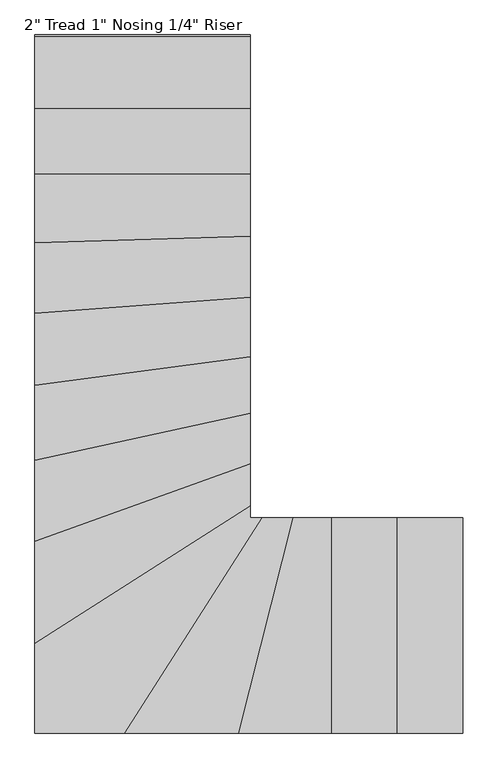
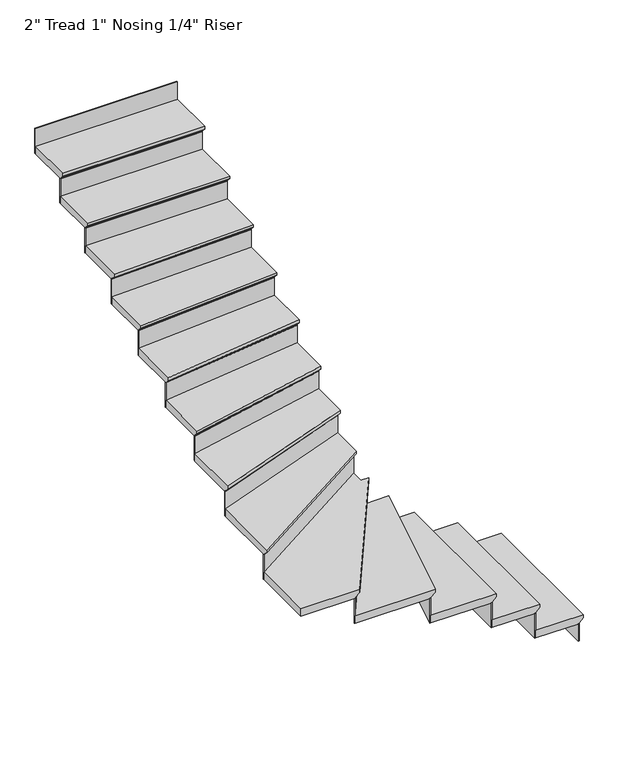
"""IFC4 building model written with IfcOpenShell, lengths in millimetres: stair flight geometry."""

from ifc_helpers import new_model, si_unit, origin, place, context, project, spatial, faceted_brep, source, transform, mapped, element, save


def stair_flight_14253777(model_context):
    return source(origin(), model_context, "Body", "Brep", [
        faceted_brep([(-4378.4230036, -1246.1564015, 10428.8166667), (-4378.4230036, -1246.1564015, 10447.8666667), (-4378.4230036, -2160.5564015, 10447.8666667), (-4378.4230036, -2160.5564015, 10428.8166667), (-4403.8230036, -1246.1564015, 10403.4166667), (-4403.8230036, -2160.5564015, 10403.4166667), (-4683.2230036, -1246.1564015, 10447.8666667), (-4683.2230036, -2160.5564015, 10447.8666667), (-4403.8230036, -2160.5564015, 10397.0666667), (-4683.2230036, -2160.5564015, 10397.0666667), (-4683.2230036, -1246.1564015, 10397.0666667), (-4403.8230036, -1246.1564015, 10397.0666667)], [[[0, 1, 2, 3]], [[4, 0, 3, 5]], [[2, 1, 6, 7]], [[8, 9, 10, 11]], [[2, 7, 9, 8, 5, 3]], [[8, 11, 4, 5]], [[6, 1, 0, 4, 11, 10]], [[7, 6, 10, 9]]]),
        faceted_brep([(-4403.8230036, -1246.1564015, 10397.0666667), (-4403.8230036, -1246.1564015, 10278.5333333), (-4410.1730036, -1246.1564015, 10278.5333333), (-4410.1730036, -1246.1564015, 10397.0666667), (-4403.8230036, -2160.5564015, 10397.0666667), (-4410.1730036, -2160.5564015, 10397.0666667), (-4410.1730036, -2160.5564015, 10278.5333333), (-4403.8230036, -2160.5564015, 10278.5333333)], [[[0, 1, 2, 3]], [[4, 5, 6, 7]], [[1, 0, 4, 7]], [[2, 1, 7, 6]], [[3, 2, 6, 5]], [[0, 3, 5, 4]]]),
        faceted_brep([(-4683.2230036, -1246.1564015, 10566.4), (-4683.2230036, -1246.1564015, 10397.0666667), (-4689.5730036, -1246.1564015, 10397.0666667), (-4689.5730036, -1246.1564015, 10566.4), (-4683.2230036, -2160.5564015, 10566.4), (-4689.5730036, -2160.5564015, 10566.4), (-4689.5730036, -2160.5564015, 10397.0666667), (-4683.2230036, -2160.5564015, 10397.0666667)], [[[0, 1, 2, 3]], [[4, 5, 6, 7]], [[1, 0, 4, 7]], [[2, 1, 7, 6]], [[3, 2, 6, 5]], [[0, 3, 5, 4]]]),
        faceted_brep([(-4657.8230036, -2160.5564015, 10617.2), (-4657.8230036, -1246.1564015, 10617.2), (-4962.6230036, -1246.1564015, 10617.2), (-4962.6230036, -2160.5564015, 10617.2), (-4683.2230036, -2160.5564015, 10566.4), (-4962.6230036, -2160.5564015, 10566.4), (-4962.6230036, -1246.1564015, 10566.4), (-4683.2230036, -1246.1564015, 10566.4), (-4683.2230036, -2160.5564015, 10572.75), (-4657.8230036, -2160.5564015, 10598.15), (-4683.2230036, -1246.1564015, 10572.75), (-4657.8230036, -1246.1564015, 10598.15)], [[[0, 1, 2, 3]], [[4, 5, 6, 7]], [[0, 3, 5, 4, 8, 9]], [[4, 7, 10, 8]], [[2, 1, 11, 10, 7, 6]], [[3, 2, 6, 5]], [[11, 1, 0, 9]], [[10, 11, 9, 8]]]),
        faceted_brep([(-4962.6230036, -1246.1564015, 10735.7333333), (-4962.6230036, -1246.1564015, 10566.4), (-4968.9730036, -1246.1564015, 10566.4), (-4968.9730036, -1246.1564015, 10735.7333333), (-4962.6230036, -2160.5564015, 10735.7333333), (-4968.9730036, -2160.5564015, 10735.7333333), (-4968.9730036, -2160.5564015, 10566.4), (-4962.6230036, -2160.5564015, 10566.4)], [[[0, 1, 2, 3]], [[4, 5, 6, 7]], [[1, 0, 4, 7]], [[2, 1, 7, 6]], [[3, 2, 6, 5]], [[0, 3, 5, 4]]]),
        faceted_brep([(-4937.2230036, -2160.5564015, 10786.5333333), (-4937.2230036, -1246.1564015, 10786.5333333), (-5127.3280374, -1246.1564015, 10786.5333333), (-5358.313714, -2160.5564015, 10786.5333333), (-4962.6230036, -2160.5564015, 10735.7333333), (-5358.313714, -2160.5564015, 10735.7333333), (-5127.3280374, -1246.1564015, 10735.7333333), (-4962.6230036, -1246.1564015, 10735.7333333), (-4962.6230036, -2160.5564015, 10742.0833333), (-4937.2230036, -2160.5564015, 10767.4833333), (-4962.6230036, -1246.1564015, 10742.0833333), (-4937.2230036, -1246.1564015, 10767.4833333)], [[[0, 1, 2, 3]], [[4, 5, 6, 7]], [[0, 3, 5, 4, 8, 9]], [[4, 7, 10, 8]], [[2, 1, 11, 10, 7, 6]], [[3, 2, 6, 5]], [[11, 1, 0, 9]], [[10, 11, 9, 8]]]),
        faceted_brep([(-5127.3280374, -1246.1564015, 10905.0666667), (-5127.3280374, -1246.1564015, 10735.7333333), (-5133.8775055, -1246.1564015, 10735.7333333), (-5133.8775055, -1246.1564015, 10905.0666667), (-5358.313714, -2160.5564015, 10905.0666667), (-5364.8631821, -2160.5564015, 10905.0666667), (-5364.8631821, -2160.5564015, 10735.7333333), (-5358.313714, -2160.5564015, 10735.7333333)], [[[0, 1, 2, 3]], [[4, 5, 6, 7]], [[1, 0, 4, 7]], [[2, 1, 7, 6]], [[3, 2, 6, 5]], [[0, 3, 5, 4]]]),
        faceted_brep([(-5332.1158419, -2160.5564015, 10955.8666667), (-5101.1301653, -1246.1564015, 10955.8666667), (-5261.5956265, -1246.1564015, 10955.8666667), (-5846.1950619, -2160.5564015, 10955.8666667), (-5358.313714, -2160.5564015, 10905.0666667), (-5846.1950619, -2160.5564015, 10905.0666667), (-5261.5956265, -1246.1564015, 10905.0666667), (-5127.3280374, -1246.1564015, 10905.0666667), (-5358.313714, -2160.5564015, 10911.4166667), (-5332.1158419, -2160.5564015, 10936.8166667), (-5127.3280374, -1246.1564015, 10911.4166667), (-5101.1301653, -1246.1564015, 10936.8166667)], [[[0, 1, 2, 3]], [[4, 5, 6, 7]], [[0, 3, 5, 4, 8, 9]], [[4, 7, 10, 8]], [[2, 1, 11, 10, 7, 6]], [[3, 2, 6, 5]], [[11, 1, 0, 9]], [[10, 11, 9, 8]]]),
        faceted_brep([(-5261.5956265, -1246.1564015, 11074.4), (-5261.5956265, -1246.1564015, 10905.0666667), (-5269.1324569, -1246.1564015, 10905.0666667), (-5269.1324569, -1246.1564015, 11074.4), (-5846.1950619, -2160.5564015, 11074.4), (-5853.7318923, -2160.5564015, 11074.4), (-5853.7318923, -2160.5564015, 10905.0666667), (-5846.1950619, -2160.5564015, 10905.0666667)], [[[0, 1, 2, 3]], [[4, 5, 6, 7]], [[1, 0, 4, 7]], [[2, 1, 7, 6]], [[3, 2, 6, 5]], [[0, 3, 5, 4]]]),
        faceted_brep([(-6196.7599931, -1749.696827, 11125.2), (-6196.7599931, -2160.5564015, 11125.2), (-5816.0477402, -2160.5564015, 11125.2), (-5231.4483048, -1246.1564015, 11125.2), (-5282.3599931, -1246.1564015, 11125.2), (-5282.3599931, -1165.0973916, 11125.2), (-6196.7599931, -2160.5564015, 11074.4), (-6196.7599931, -1749.696827, 11074.4), (-5282.3599931, -1165.0973916, 11074.4), (-5282.3599931, -1246.1564015, 11074.4), (-5261.5956265, -1246.1564015, 11074.4), (-5846.1950619, -2160.5564015, 11074.4), (-5261.5956265, -1246.1564015, 11080.75), (-5846.1950619, -2160.5564015, 11080.75), (-5231.4483048, -1246.1564015, 11106.15), (-5816.0477402, -2160.5564015, 11106.15)], [[[0, 1, 2, 3, 4, 5]], [[6, 7, 8, 9, 10, 11]], [[1, 0, 7, 6]], [[11, 10, 12, 13]], [[4, 3, 14, 12, 10, 9]], [[0, 5, 8, 7]], [[14, 3, 2, 15]], [[12, 14, 15, 13]], [[2, 1, 6, 11, 13, 15]], [[5, 4, 9, 8]]]),
        faceted_brep([(-5282.3599931, -1165.0973916, 11243.7333333), (-5282.3599931, -1165.0973916, 11074.4), (-5282.3599931, -1157.5605612, 11074.4), (-5282.3599931, -1157.5605612, 11243.7333333), (-6196.7599931, -1749.696827, 11243.7333333), (-6196.7599931, -1742.1599966, 11243.7333333), (-6196.7599931, -1742.1599966, 11074.4), (-6196.7599931, -1749.696827, 11074.4)], [[[0, 1, 2, 3]], [[4, 5, 6, 7]], [[1, 0, 4, 7]], [[2, 1, 7, 6]], [[3, 2, 6, 5]], [[0, 3, 5, 4]]]),
        faceted_brep([(-6196.7599931, -1779.8441487, 11294.5333333), (-5282.3599931, -1195.2447133, 11294.5333333), (-5282.3599931, -989.1410797, 11294.5333333), (-6196.7599931, -1317.7175845, 11294.5333333), (-6196.7599931, -1749.696827, 11243.7333333), (-6196.7599931, -1317.7175845, 11243.7333333), (-5282.3599931, -989.1410797, 11243.7333333), (-5282.3599931, -1165.0973916, 11243.7333333), (-6196.7599931, -1749.696827, 11250.0833333), (-6196.7599931, -1779.8441487, 11275.4833333), (-5282.3599931, -1165.0973916, 11250.0833333), (-5282.3599931, -1195.2447133, 11275.4833333)], [[[0, 1, 2, 3]], [[4, 5, 6, 7]], [[0, 3, 5, 4, 8, 9]], [[4, 7, 10, 8]], [[2, 1, 11, 10, 7, 6]], [[3, 2, 6, 5]], [[11, 1, 0, 9]], [[10, 11, 9, 8]]]),
        faceted_brep([(-5282.3599931, -989.1410797, 11413.0666667), (-5282.3599931, -989.1410797, 11243.7333333), (-5282.3599931, -982.3935597, 11243.7333333), (-5282.3599931, -982.3935597, 11413.0666667), (-6196.7599931, -1317.7175845, 11413.0666667), (-6196.7599931, -1310.9700645, 11413.0666667), (-6196.7599931, -1310.9700645, 11243.7333333), (-6196.7599931, -1317.7175845, 11243.7333333)], [[[0, 1, 2, 3]], [[4, 5, 6, 7]], [[1, 0, 4, 7]], [[2, 1, 7, 6]], [[3, 2, 6, 5]], [[0, 3, 5, 4]]]),
        faceted_brep([(-6196.7599931, -1344.7076644, 11463.8666667), (-5282.3599931, -1016.1311596, 11463.8666667), (-5282.3599931, -775.0246806, 11463.8666667), (-6196.7599931, -975.0133472, 11463.8666667), (-6196.7599931, -1317.7175845, 11413.0666667), (-6196.7599931, -975.0133472, 11413.0666667), (-5282.3599931, -775.0246806, 11413.0666667), (-5282.3599931, -989.1410797, 11413.0666667), (-6196.7599931, -1317.7175845, 11419.4166667), (-6196.7599931, -1344.7076644, 11444.8166667), (-5282.3599931, -989.1410797, 11419.4166667), (-5282.3599931, -1016.1311596, 11444.8166667)], [[[0, 1, 2, 3]], [[4, 5, 6, 7]], [[0, 3, 5, 4, 8, 9]], [[4, 7, 10, 8]], [[2, 1, 11, 10, 7, 6]], [[3, 2, 6, 5]], [[11, 1, 0, 9]], [[10, 11, 9, 8]]]),
        faceted_brep([(-5282.3599931, -775.0246806, 11582.4), (-5282.3599931, -775.0246806, 11413.0666667), (-5282.3599931, -768.5245811, 11413.0666667), (-5282.3599931, -768.5245811, 11582.4), (-6196.7599931, -975.0133472, 11582.4), (-6196.7599931, -968.5132477, 11582.4), (-6196.7599931, -968.5132477, 11413.0666667), (-6196.7599931, -975.0133472, 11413.0666667)], [[[0, 1, 2, 3]], [[4, 5, 6, 7]], [[1, 0, 4, 7]], [[2, 1, 7, 6]], [[3, 2, 6, 5]], [[0, 3, 5, 4]]]),
        faceted_brep([(-6196.7599931, -1001.0137453, 11633.2), (-5282.3599931, -801.0250787, 11633.2), (-5282.3599931, -535.4776405, 11633.2), (-6196.7599931, -656.5180526, 11633.2), (-6196.7599931, -975.0133472, 11582.4), (-6196.7599931, -656.5180526, 11582.4), (-5282.3599931, -535.4776405, 11582.4), (-5282.3599931, -775.0246806, 11582.4), (-6196.7599931, -975.0133472, 11588.75), (-6196.7599931, -1001.0137453, 11614.15), (-5282.3599931, -775.0246806, 11588.75), (-5282.3599931, -801.0250787, 11614.15)], [[[0, 1, 2, 3]], [[4, 5, 6, 7]], [[0, 3, 5, 4, 8, 9]], [[4, 7, 10, 8]], [[2, 1, 11, 10, 7, 6]], [[3, 2, 6, 5]], [[11, 1, 0, 9]], [[10, 11, 9, 8]]]),
        faceted_brep([(-5282.3599931, -535.4776405, 11751.7333333), (-5282.3599931, -535.4776405, 11582.4), (-5282.3599931, -529.0722492, 11582.4), (-5282.3599931, -529.0722492, 11751.7333333), (-6196.7599931, -656.5180526, 11751.7333333), (-6196.7599931, -650.1126613, 11751.7333333), (-6196.7599931, -650.1126613, 11582.4), (-6196.7599931, -656.5180526, 11582.4)], [[[0, 1, 2, 3]], [[4, 5, 6, 7]], [[1, 0, 4, 7]], [[2, 1, 7, 6]], [[3, 2, 6, 5]], [[0, 3, 5, 4]]]),
        faceted_brep([(-6196.7599931, -682.139618, 11802.5333333), (-5282.3599931, -561.099206, 11802.5333333), (-5282.3599931, -282.9309158, 11802.5333333), (-6196.7599931, -350.56912, 11802.5333333), (-6196.7599931, -656.5180526, 11751.7333333), (-6196.7599931, -350.56912, 11751.7333333), (-5282.3599931, -282.9309158, 11751.7333333), (-5282.3599931, -535.4776405, 11751.7333333), (-6196.7599931, -656.5180526, 11758.0833333), (-6196.7599931, -682.139618, 11783.4833333), (-5282.3599931, -535.4776405, 11758.0833333), (-5282.3599931, -561.099206, 11783.4833333)], [[[0, 1, 2, 3]], [[4, 5, 6, 7]], [[0, 3, 5, 4, 8, 9]], [[4, 7, 10, 8]], [[2, 1, 11, 10, 7, 6]], [[3, 2, 6, 5]], [[11, 1, 0, 9]], [[10, 11, 9, 8]]]),
        faceted_brep([(-5282.3599931, -282.9309158, 11921.0666667), (-5282.3599931, -282.9309158, 11751.7333333), (-5282.3599931, -276.5635673, 11751.7333333), (-5282.3599931, -276.5635673, 11921.0666667), (-6196.7599931, -350.56912, 11921.0666667), (-6196.7599931, -344.2017715, 11921.0666667), (-6196.7599931, -344.2017715, 11751.7333333), (-6196.7599931, -350.56912, 11751.7333333)], [[[0, 1, 2, 3]], [[4, 5, 6, 7]], [[1, 0, 4, 7]], [[2, 1, 7, 6]], [[3, 2, 6, 5]], [[0, 3, 5, 4]]]),
        faceted_brep([(-6196.7599931, -376.0385141, 11971.8666667), (-5282.3599931, -308.4003099, 11971.8666667), (-5282.3599931, -22.8518026, 11971.8666667), (-6196.7599931, -51.9612867, 11971.8666667), (-6196.7599931, -350.56912, 11921.0666667), (-6196.7599931, -51.9612867, 11921.0666667), (-5282.3599931, -22.8518026, 11921.0666667), (-5282.3599931, -282.9309158, 11921.0666667), (-6196.7599931, -350.56912, 11927.4166667), (-6196.7599931, -376.0385141, 11952.8166667), (-5282.3599931, -282.9309158, 11927.4166667), (-5282.3599931, -308.4003099, 11952.8166667)], [[[0, 1, 2, 3]], [[4, 5, 6, 7]], [[0, 3, 5, 4, 8, 9]], [[4, 7, 10, 8]], [[2, 1, 11, 10, 7, 6]], [[3, 2, 6, 5]], [[11, 1, 0, 9]], [[10, 11, 9, 8]]]),
        faceted_brep([(-5282.3599931, -22.8518026, 12090.4), (-5282.3599931, -22.8518026, 11921.0666667), (-5282.3599931, -16.4985857, 11921.0666667), (-5282.3599931, -16.4985857, 12090.4), (-6196.7599931, -51.9612867, 12090.4), (-6196.7599931, -45.6080698, 12090.4), (-6196.7599931, -45.6080698, 11921.0666667), (-6196.7599931, -51.9612867, 11921.0666667)], [[[0, 1, 2, 3]], [[4, 5, 6, 7]], [[1, 0, 4, 7]], [[2, 1, 7, 6]], [[3, 2, 6, 5]], [[0, 3, 5, 4]]]),
        faceted_brep([(-6196.7599931, -77.3741541, 12141.2), (-5282.3599931, -48.26467, 12141.2), (-5282.3599931, 241.980588, 12141.2), (-6196.7599931, 241.980588, 12141.2), (-6196.7599931, -51.9612867, 12090.4), (-6196.7599931, 241.980588, 12090.4), (-5282.3599931, 241.980588, 12090.4), (-5282.3599931, -22.8518026, 12090.4), (-6196.7599931, -51.9612867, 12096.75), (-6196.7599931, -77.3741541, 12122.15), (-5282.3599931, -22.8518026, 12096.75), (-5282.3599931, -48.26467, 12122.15)], [[[0, 1, 2, 3]], [[4, 5, 6, 7]], [[0, 3, 5, 4, 8, 9]], [[4, 7, 10, 8]], [[2, 1, 11, 10, 7, 6]], [[3, 2, 6, 5]], [[11, 1, 0, 9]], [[10, 11, 9, 8]]]),
        faceted_brep([(-5282.3599931, 241.980588, 12259.7333333), (-5282.3599931, 241.980588, 12090.4), (-5282.3599931, 248.330588, 12090.4), (-5282.3599931, 248.330588, 12259.7333333), (-6196.7599931, 241.980588, 12259.7333333), (-6196.7599931, 248.330588, 12259.7333333), (-6196.7599931, 248.330588, 12090.4), (-6196.7599931, 241.980588, 12090.4)], [[[0, 1, 2, 3]], [[4, 5, 6, 7]], [[1, 0, 4, 7]], [[2, 1, 7, 6]], [[3, 2, 6, 5]], [[0, 3, 5, 4]]]),
        faceted_brep([(-6196.7599931, 216.580588, 12310.5333333), (-5282.3599931, 216.580588, 12310.5333333), (-5282.3599931, 521.380588, 12310.5333333), (-6196.7599931, 521.380588, 12310.5333333), (-6196.7599931, 241.980588, 12259.7333333), (-6196.7599931, 521.380588, 12259.7333333), (-5282.3599931, 521.380588, 12259.7333333), (-5282.3599931, 241.980588, 12259.7333333), (-6196.7599931, 241.980588, 12266.0833333), (-6196.7599931, 216.580588, 12291.4833333), (-5282.3599931, 241.980588, 12266.0833333), (-5282.3599931, 216.580588, 12291.4833333)], [[[0, 1, 2, 3]], [[4, 5, 6, 7]], [[0, 3, 5, 4, 8, 9]], [[4, 7, 10, 8]], [[2, 1, 11, 10, 7, 6]], [[3, 2, 6, 5]], [[11, 1, 0, 9]], [[10, 11, 9, 8]]]),
        faceted_brep([(-5282.3599931, 521.380588, 12429.0666667), (-5282.3599931, 521.380588, 12259.7333333), (-5282.3599931, 527.730588, 12259.7333333), (-5282.3599931, 527.730588, 12429.0666667), (-6196.7599931, 521.380588, 12429.0666667), (-6196.7599931, 527.730588, 12429.0666667), (-6196.7599931, 527.730588, 12259.7333333), (-6196.7599931, 521.380588, 12259.7333333)], [[[0, 1, 2, 3]], [[4, 5, 6, 7]], [[1, 0, 4, 7]], [[2, 1, 7, 6]], [[3, 2, 6, 5]], [[0, 3, 5, 4]]]),
        faceted_brep([(-5282.3599931, 800.780588, 12598.4), (-5282.3599931, 800.780588, 12429.0666667), (-5282.3599931, 807.130588, 12429.0666667), (-5282.3599931, 807.130588, 12598.4), (-6196.7599931, 800.780588, 12598.4), (-6196.7599931, 807.130588, 12598.4), (-6196.7599931, 807.130588, 12429.0666667), (-6196.7599931, 800.780588, 12429.0666667)], [[[0, 1, 2, 3]], [[4, 5, 6, 7]], [[1, 0, 4, 7]], [[2, 1, 7, 6]], [[3, 2, 6, 5]], [[0, 3, 5, 4]]]),
        faceted_brep([(-6196.7599931, 495.980588, 12479.8666667), (-5282.3599931, 495.980588, 12479.8666667), (-5282.3599931, 800.780588, 12479.8666667), (-6196.7599931, 800.780588, 12479.8666667), (-6196.7599931, 521.380588, 12429.0666667), (-6196.7599931, 800.780588, 12429.0666667), (-5282.3599931, 800.780588, 12429.0666667), (-5282.3599931, 521.380588, 12429.0666667), (-6196.7599931, 521.380588, 12435.4166667), (-6196.7599931, 495.980588, 12460.8166667), (-5282.3599931, 521.380588, 12435.4166667), (-5282.3599931, 495.980588, 12460.8166667)], [[[0, 1, 2, 3]], [[4, 5, 6, 7]], [[0, 3, 5, 4, 8, 9]], [[4, 7, 10, 8]], [[2, 1, 11, 10, 7, 6]], [[3, 2, 6, 5]], [[11, 1, 0, 9]], [[10, 11, 9, 8]]]),
    ])


if __name__ == "__main__":
    model = new_model("IFC4")
    model_context = context("Model", 3, world=origin())
    ifc_project = project(units=[si_unit("LENGTHUNIT", "METRE", prefix="MILLI")], contexts=[model_context])
    site = spatial("IfcSite", under=ifc_project)
    building = spatial("IfcBuilding", under=site)
    placement = place(None, origin())
    stair_flight_shape = stair_flight_14253777(model_context)
    element("IfcStairFlight", 1, ObjectType="2\" Tread 1\" Nosing 1/4\" Riser", at=placement, inside=building, context=model_context, shape_type="MappedRepresentation", body=[
        mapped(stair_flight_shape, transform((0.0, 0.0, 0.0), x_axis=(1.0, 0.0, 0.0), y_axis=(0.0, 1.0, 0.0), z_axis=(0.0, 0.0, 1.0))),
    ])
    save(model, "model.ifc")
